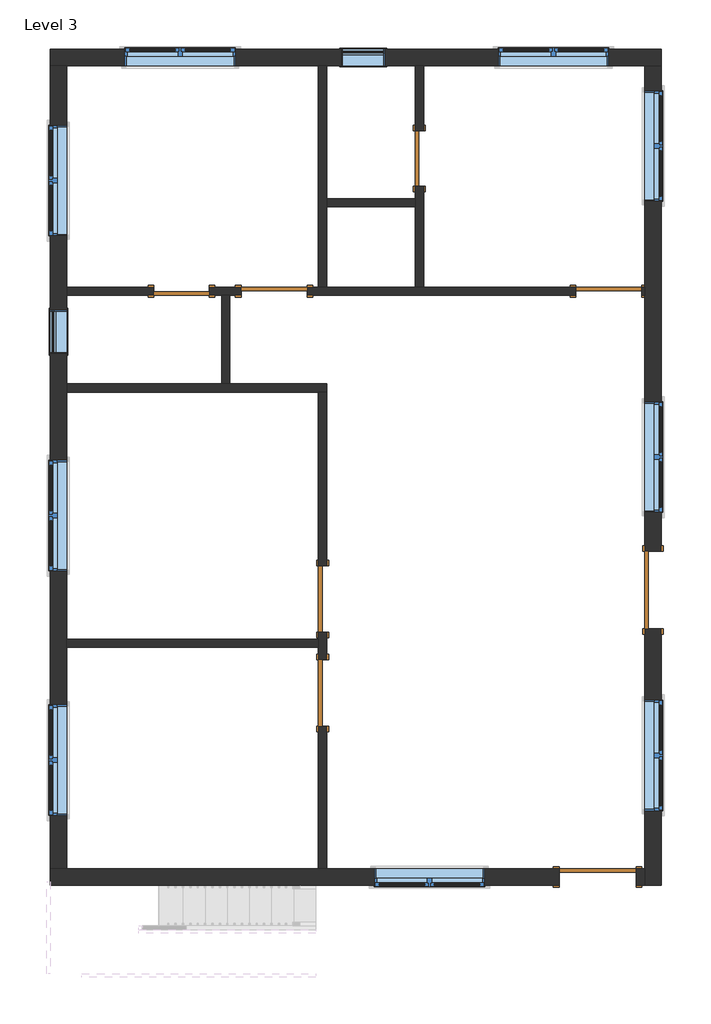
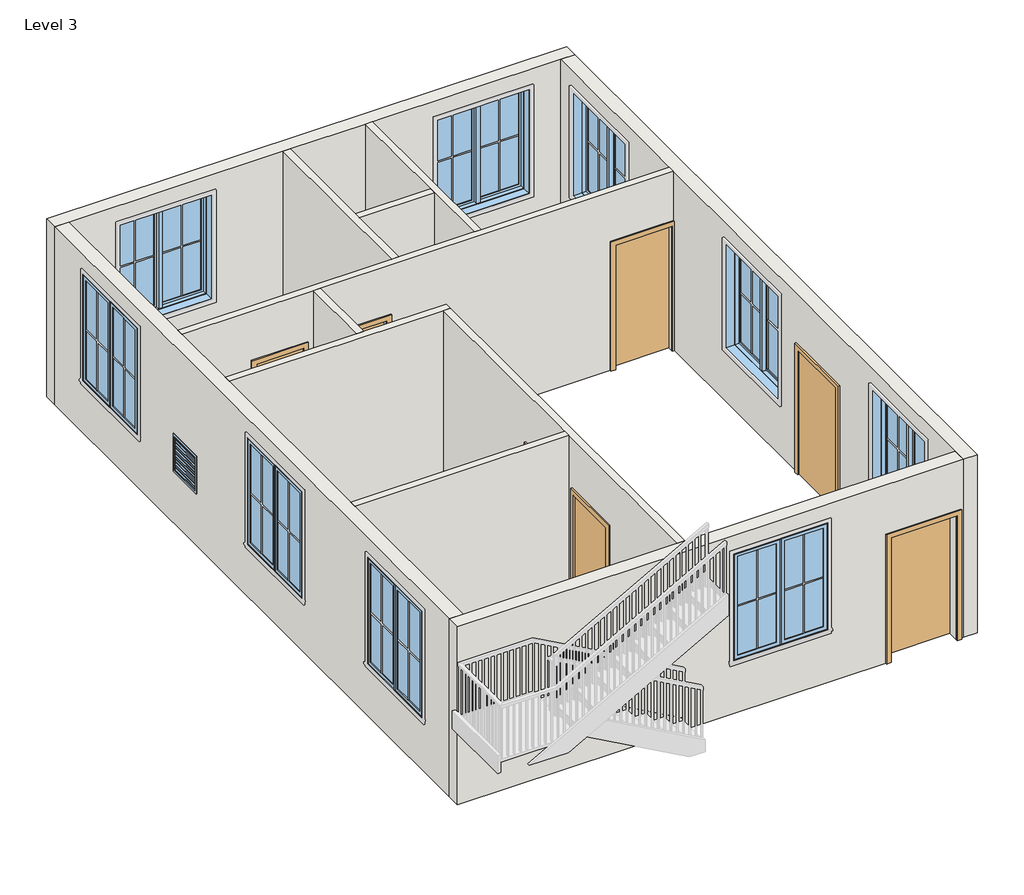
# One storey, part 1 of 3: 12 walls, 11 windows, 8 doors.
"""IFC4 building model written with IfcOpenShell, lengths in millimetres."""

from ifc_helpers import new_model, si_unit, frame, origin, place, context, project, spatial, polyline, outline, extrude, faceted_brep, transform, mapped, element, save
from components import door_78caadf7, single_flush_door_3_e5f9f3c4, single_flush_door_3_305aa2a5, door_9d399b00, door_0848dd25, window_casement_double_win_5_f93960c7, window_f2d8fef0

model = new_model("IFC4")

# Units and contexts
model_context = context("Model", 3, world=origin())
ifc_project = project(units=[si_unit("LENGTHUNIT", "METRE", prefix="MILLI")], contexts=[model_context])

# Site, building, storey
site = spatial("IfcSite", under=ifc_project)
building = spatial("IfcBuilding", under=site)
storey = spatial("IfcBuildingStorey", under=building, Name="Level 3", Elevation=3200.4)

# Doors
placement = place(None, origin())
door_shape = door_78caadf7(model_context)
element("IfcDoor", 1, ObjectType="Single-Flush : DOOR 2'6\"", at=placement, inside=storey, context=model_context, shape_type="MappedRepresentation", body=[
    mapped(door_shape, transform((-377.1698569, 4707.5566963, 3200.4), x_axis=(0.0, -1.0, 0.0), y_axis=(1.0, 0.0, 0.0), z_axis=(0.0, 0.0, 1.0))),
])
element("IfcDoor", 2, ObjectType="Single-Flush : DOOR 2'6\"", at=placement, inside=storey, context=model_context, shape_type="MappedRepresentation", body=[
    mapped(door_shape, transform((-3653.7698569, 2878.7566963, 3200.4), x_axis=(1.0, 0.0, 0.0), y_axis=(0.0, 1.0, 0.0), z_axis=(0.0, 0.0, 1.0))),
])
single_flush_door_3_shape = single_flush_door_3_e5f9f3c4(model_context)
element("IfcDoor", 3, ObjectType="Single-Flush : DOOR 3'", at=placement, inside=storey, context=model_context, shape_type="MappedRepresentation", body=[
    mapped(single_flush_door_3_shape, transform((-2377.4198569, 2878.7566963, 3200.4), x_axis=(1.0, 0.0, 0.0), y_axis=(0.0, 1.0, 0.0), z_axis=(0.0, 0.0, 1.0))),
])
element("IfcDoor", 4, ObjectType="Single-Flush : DOOR 3'", at=placement, inside=storey, context=model_context, shape_type="MappedRepresentation", body=[
    mapped(single_flush_door_3_shape, transform((2232.6801431, 2878.7566963, 3200.4), x_axis=(1.0, 0.0, 0.0), y_axis=(0.0, 1.0, 0.0), z_axis=(0.0, 0.0, 1.0))),
])
element("IfcDoor", 5, ObjectType="Single-Flush : DOOR 3'", at=placement, inside=storey, context=model_context, shape_type="MappedRepresentation", body=[
    mapped(single_flush_door_3_shape, transform((-1710.6698569, -2658.4433037, 3200.4), x_axis=(0.0, 1.0, 0.0), y_axis=(-1.0, 0.0, 0.0), z_axis=(0.0, 0.0, 1.0))),
])
single_flush_door_3_2_shape = single_flush_door_3_305aa2a5(model_context)
element("IfcDoor", 6, ObjectType="Single-Flush : DOOR 3'", at=placement, inside=storey, context=model_context, shape_type="MappedRepresentation", body=[
    mapped(single_flush_door_3_2_shape, transform((-1710.6698569, -1363.0433037, 3200.4), x_axis=(0.0, -1.0, 0.0), y_axis=(1.0, 0.0, 0.0), z_axis=(0.0, 0.0, 1.0))),
])
door_2_shape = door_9d399b00(model_context)
element("IfcDoor", 7, ObjectType="Single-Flush : DOOR 3'6\"", at=placement, inside=storey, context=model_context, shape_type="MappedRepresentation", body=[
    mapped(door_2_shape, transform((2080.2801431, -5192.0933037, 3200.4), x_axis=(1.0, 0.0, 0.0), y_axis=(0.0, 1.0, 0.0), z_axis=(0.0, 0.0, 1.0))),
])
door_3_shape = door_0848dd25(model_context)
element("IfcDoor", 8, ObjectType="Single-Flush : DOOR 3'6\"", at=placement, inside=storey, context=model_context, shape_type="MappedRepresentation", body=[
    mapped(door_3_shape, transform((2842.2801431, -1236.0433037, 3200.4), x_axis=(0.0, -1.0, 0.0), y_axis=(1.0, 0.0, 0.0), z_axis=(0.0, 0.0, 1.0))),
])

# Walls
element("IfcWall", 9, ObjectType="WALL 4.5\"", at=placement, inside=storey, context=model_context, shape_type="Brep", body=[
    faceted_brep([(2689.8801431, 2821.6066963, 5334.0), (2689.8801431, 2821.6066963, 3200.4), (2727.9801431, 2821.6066963, 3200.4), (2727.9801431, 2821.6066963, 6248.4), (-2987.0198569, 2821.6066963, 6248.4), (-3101.3198569, 2821.6066963, 6248.4), (-5234.9198569, 2821.6066963, 6248.4), (-5234.9198569, 2821.6066963, 3200.4), (-4034.7698569, 2821.6066963, 3200.4), (-4034.7698569, 2821.6066963, 5334.0), (-3272.7698569, 2821.6066963, 5334.0), (-3272.7698569, 2821.6066963, 3200.4), (-3101.3198569, 2821.6066963, 3200.4), (-2987.0198569, 2821.6066963, 3200.4), (-2834.6198569, 2821.6066963, 3200.4), (-2834.6198569, 2821.6066963, 5334.0), (-1920.2198569, 2821.6066963, 5334.0), (-1920.2198569, 2821.6066963, 3200.4), (1775.4801431, 2821.6066963, 3200.4), (1775.4801431, 2821.6066963, 5334.0), (2727.9801431, 2935.9066963, 3200.4), (2689.8801431, 2935.9066963, 3200.4), (2689.8801431, 2935.9066963, 5334.0), (1775.4801431, 2935.9066963, 5334.0), (1775.4801431, 2935.9066963, 3200.4), (-320.0198569, 2935.9066963, 3200.4), (-434.3198569, 2935.9066963, 3200.4), (-1653.5198569, 2935.9066963, 3200.4), (-1767.8198569, 2935.9066963, 3200.4), (-1920.2198569, 2935.9066963, 3200.4), (-1920.2198569, 2935.9066963, 5334.0), (-2834.6198569, 2935.9066963, 5334.0), (-2834.6198569, 2935.9066963, 3200.4), (-3272.7698569, 2935.9066963, 3200.4), (-3272.7698569, 2935.9066963, 5334.0), (-4034.7698569, 2935.9066963, 5334.0), (-4034.7698569, 2935.9066963, 3200.4), (-5234.9198569, 2935.9066963, 3200.4), (-5234.9198569, 2935.9066963, 6248.4), (-1767.8198569, 2935.9066963, 6248.4), (-1653.5198569, 2935.9066963, 6248.4), (-434.3198569, 2935.9066963, 6248.4), (-320.0198569, 2935.9066963, 6248.4), (2727.9801431, 2935.9066963, 6248.4)], [[[0, 1, 2, 3, 4, 5, 6, 7, 8, 9, 10, 11, 12, 13, 14, 15, 16, 17, 18, 19]], [[20, 21, 22, 23, 24, 25, 26, 27, 28, 29, 30, 31, 32, 33, 34, 35, 36, 37, 38, 39, 40, 41, 42, 43]], [[8, 7, 37, 36]], [[14, 13, 12, 11, 33, 32]], [[18, 17, 29, 28, 27, 26, 25, 24]], [[2, 1, 21, 20]], [[3, 2, 20, 43]], [[7, 6, 38, 37]], [[34, 33, 11, 10]], [[35, 34, 10, 9]], [[36, 35, 9, 8]], [[30, 29, 17, 16]], [[31, 30, 16, 15]], [[32, 31, 15, 14]], [[22, 21, 1, 0]], [[23, 22, 0, 19]], [[24, 23, 19, 18]], [[6, 5, 4, 3, 43, 42, 41, 40, 39, 38]]]),
])
element("IfcWall", 10, ObjectType="WALL 4.5\"", at=placement, inside=storey, context=model_context, shape_type="Brep", body=[
    faceted_brep([(-1767.8198569, 5983.9066963, 3200.4), (-1767.8198569, 2935.9066963, 3200.4), (-1767.8198569, 2935.9066963, 6248.4), (-1767.8198569, 5983.9066963, 6248.4), (-1653.5198569, 5983.9066963, 3200.4), (-1653.5198569, 5983.9066963, 6248.4), (-1653.5198569, 4155.1066963, 6248.4), (-1653.5198569, 4040.8066963, 6248.4), (-1653.5198569, 2935.9066963, 6248.4), (-1653.5198569, 2935.9066963, 3200.4), (-1653.5198569, 4040.8066963, 3200.4), (-1653.5198569, 4155.1066963, 3200.4)], [[[0, 1, 2, 3]], [[4, 5, 6, 7, 8, 9, 10, 11]], [[1, 0, 4, 11, 10, 9]], [[0, 3, 5, 4]], [[2, 1, 9, 8]], [[3, 2, 8, 7, 6, 5]]]),
])
element("IfcWall", 11, ObjectType="WALL 4.5\"", at=placement, inside=storey, context=model_context, shape_type="Brep", body=[
    faceted_brep([(-320.0198569, 2935.9066963, 3200.4), (-320.0198569, 4326.5566963, 3200.4), (-320.0198569, 4326.5566963, 5334.0), (-320.0198569, 5088.5566963, 5334.0), (-320.0198569, 5088.5566963, 3200.4), (-320.0198569, 5983.9066963, 3200.4), (-320.0198569, 5983.9066963, 6248.4), (-320.0198569, 2935.9066963, 6248.4), (-434.3198569, 4326.5566963, 5334.0), (-434.3198569, 4326.5566963, 3200.4), (-434.3198569, 4155.1066963, 3200.4), (-434.3198569, 4040.8066963, 3200.4), (-434.3198569, 2935.9066963, 3200.4), (-434.3198569, 2935.9066963, 6248.4), (-434.3198569, 4040.8066963, 6248.4), (-434.3198569, 4155.1066963, 6248.4), (-434.3198569, 5983.9066963, 6248.4), (-434.3198569, 5983.9066963, 3200.4), (-434.3198569, 5088.5566963, 3200.4), (-434.3198569, 5088.5566963, 5334.0)], [[[0, 1, 2, 3, 4, 5, 6, 7]], [[8, 9, 10, 11, 12, 13, 14, 15, 16, 17, 18, 19]], [[18, 17, 5, 4]], [[12, 11, 10, 9, 1, 0]], [[6, 5, 17, 16]], [[0, 7, 13, 12]], [[2, 1, 9, 8]], [[3, 2, 8, 19]], [[4, 3, 19, 18]], [[7, 6, 16, 15, 14, 13]]]),
])
element("IfcWall", 12, ObjectType="WALL 4.5\"", at=placement, inside=storey, context=model_context, shape_type="SweptSolid", body=[
    extrude(outline(polyline([(-434.3198569, 4040.8066963), (-1653.5198569, 4040.8066963), (-1653.5198569, 4155.1066963), (-434.3198569, 4155.1066963), (-434.3198569, 4040.8066963)])), frame((0.0, 0.0, 3200.4), z_axis=(0.0, 0.0, 1.0), x_axis=(1.0, 0.0, 0.0)), (0.0, 0.0, 1.0), 3048.0),
])
element("IfcWall", 13, ObjectType="WALL 4.5\"", at=placement, inside=storey, context=model_context, shape_type="Brep", body=[
    faceted_brep([(-5234.9198569, 1488.1066963, 3200.4), (-1767.8198569, 1488.1066963, 3200.4), (-1653.5198569, 1488.1066963, 3200.4), (-1653.5198569, 1488.1066963, 6248.4), (-1767.8198569, 1488.1066963, 6248.4), (-5234.9198569, 1488.1066963, 6248.4), (-5234.9198569, 1602.4066963, 3200.4), (-5234.9198569, 1602.4066963, 6248.4), (-3101.3198569, 1602.4066963, 6248.4), (-2987.0198569, 1602.4066963, 6248.4), (-1653.5198569, 1602.4066963, 6248.4), (-1653.5198569, 1602.4066963, 3200.4), (-2987.0198569, 1602.4066963, 3200.4), (-3101.3198569, 1602.4066963, 3200.4)], [[[0, 1, 2, 3, 4, 5]], [[6, 7, 8, 9, 10, 11, 12, 13]], [[2, 1, 0, 6, 13, 12, 11]], [[0, 5, 7, 6]], [[3, 2, 11, 10]], [[5, 4, 3, 10, 9, 8, 7]]]),
])
element("IfcWall", 14, ObjectType="WALL 4.5\"", at=placement, inside=storey, context=model_context, shape_type="Brep", body=[
    faceted_brep([(-1767.8198569, -1820.2433037, 3200.4), (-1767.8198569, -1915.4933037, 3200.4), (-1767.8198569, -2029.7933037, 3200.4), (-1767.8198569, -2201.2433037, 3200.4), (-1767.8198569, -2201.2433037, 5334.0), (-1767.8198569, -3115.6433037, 5334.0), (-1767.8198569, -3115.6433037, 3200.4), (-1767.8198569, -5077.7933037, 3200.4), (-1767.8198569, -5077.7933037, 6248.4), (-1767.8198569, -2029.7933037, 6248.4), (-1767.8198569, -1915.4933037, 6248.4), (-1767.8198569, 1488.1066963, 6248.4), (-1767.8198569, 1488.1066963, 3200.4), (-1767.8198569, -905.8433037, 3200.4), (-1767.8198569, -905.8433037, 5334.0), (-1767.8198569, -1820.2433037, 5334.0), (-1653.5198569, -2201.2433037, 5334.0), (-1653.5198569, -2201.2433037, 3200.4), (-1653.5198569, -1820.2433037, 3200.4), (-1653.5198569, -1820.2433037, 5334.0), (-1653.5198569, -905.8433037, 5334.0), (-1653.5198569, -905.8433037, 3200.4), (-1653.5198569, 1488.1066963, 3200.4), (-1653.5198569, 1488.1066963, 6248.4), (-1653.5198569, -5077.7933037, 6248.4), (-1653.5198569, -5077.7933037, 3200.4), (-1653.5198569, -3115.6433037, 3200.4), (-1653.5198569, -3115.6433037, 5334.0)], [[[0, 1, 2, 3, 4, 5, 6, 7, 8, 9, 10, 11, 12, 13, 14, 15]], [[16, 17, 18, 19, 20, 21, 22, 23, 24, 25, 26, 27]], [[13, 12, 22, 21]], [[26, 25, 7, 6]], [[18, 17, 3, 2, 1, 0]], [[12, 11, 23, 22]], [[8, 7, 25, 24]], [[19, 18, 0, 15]], [[20, 19, 15, 14]], [[21, 20, 14, 13]], [[4, 3, 17, 16]], [[5, 4, 16, 27]], [[6, 5, 27, 26]], [[11, 10, 9, 8, 24, 23]]]),
])
element("IfcWall", 15, ObjectType="WALL 4.5\"", at=placement, inside=storey, context=model_context, shape_type="SweptSolid", body=[
    extrude(outline(polyline([(-1767.8198569, -2029.7933037), (-5234.9198569, -2029.7933037), (-5234.9198569, -1915.4933037), (-1767.8198569, -1915.4933037), (-1767.8198569, -2029.7933037)])), frame((0.0, 0.0, 3200.4), z_axis=(0.0, 0.0, 1.0), x_axis=(1.0, 0.0, 0.0)), (0.0, 0.0, 1.0), 3048.0),
])
element("IfcWall", 16, ObjectType="WALL 4.5\"", at=placement, inside=storey, context=model_context, shape_type="SweptSolid", body=[
    extrude(outline(polyline([(-3101.3198569, 1602.4066963), (-3101.3198569, 2821.6066963), (-2987.0198569, 2821.6066963), (-2987.0198569, 1602.4066963), (-3101.3198569, 1602.4066963)])), frame((0.0, 0.0, 3200.4), z_axis=(0.0, 0.0, 1.0), x_axis=(1.0, 0.0, 0.0)), (0.0, 0.0, 1.0), 3048.0),
])
element("IfcWall", 17, ObjectType="WALL 9\"", at=placement, inside=storey, context=model_context, shape_type="Brep", body=[
    faceted_brep([(-5463.5198569, 5983.9066963, 3200.4), (-5234.9198569, 5983.9066963, 3200.4), (-1767.8198569, 5983.9066963, 3200.4), (-1653.5198569, 5983.9066963, 3200.4), (-434.3198569, 5983.9066963, 3200.4), (-320.0198569, 5983.9066963, 3200.4), (2727.9801431, 5983.9066963, 3200.4), (2956.5801431, 5983.9066963, 3200.4), (2956.5801431, 5983.9066963, 6248.4), (2727.9801431, 5983.9066963, 6248.4), (-320.0198569, 5983.9066963, 6248.4), (-434.3198569, 5983.9066963, 6248.4), (-1653.5198569, 5983.9066963, 6248.4), (-1767.8198569, 5983.9066963, 6248.4), (-5234.9198569, 5983.9066963, 6248.4), (-5463.5198569, 5983.9066963, 6248.4), (2232.6801431, 5983.9066963, 5943.6), (2232.6801431, 5983.9066963, 4114.8), (708.6801431, 5983.9066963, 4114.8), (708.6801431, 5983.9066963, 5943.6), (-2910.8198569, 5983.9066963, 5943.6), (-2910.8198569, 5983.9066963, 4114.8), (-4434.8198569, 5983.9066963, 4114.8), (-4434.8198569, 5983.9066963, 5943.6), (-1456.6698569, 5983.9066963, 4724.4), (-847.0698569, 5983.9066963, 4724.4), (-847.0698569, 5983.9066963, 4114.8), (-1456.6698569, 5983.9066963, 4114.8), (-5463.5198569, 6212.5066963, 3200.4), (-5463.5198569, 6212.5066963, 6248.4), (2956.5801431, 6212.5066963, 6248.4), (2956.5801431, 6212.5066963, 3200.4), (2232.6801431, 6212.5066963, 5943.6), (708.6801431, 6212.5066963, 5943.6), (708.6801431, 6212.5066963, 4114.8), (2232.6801431, 6212.5066963, 4114.8), (-2910.8198569, 6212.5066963, 5943.6), (-4434.8198569, 6212.5066963, 5943.6), (-4434.8198569, 6212.5066963, 4114.8), (-2910.8198569, 6212.5066963, 4114.8), (-1456.6698569, 6212.5066963, 4724.4), (-1456.6698569, 6212.5066963, 4114.8), (-847.0698569, 6212.5066963, 4114.8), (-847.0698569, 6212.5066963, 4724.4)], [[[0, 1, 2, 3, 4, 5, 6, 7, 8, 9, 10, 11, 12, 13, 14, 15], [16, 17, 18, 19], [20, 21, 22, 23], [24, 25, 26, 27]], [[28, 29, 30, 31], [32, 33, 34, 35], [36, 37, 38, 39], [40, 41, 42, 43]], [[7, 6, 5, 4, 3, 2, 1, 0, 28, 31]], [[8, 7, 31, 30]], [[0, 15, 29, 28]], [[17, 16, 32, 35]], [[18, 17, 35, 34]], [[19, 18, 34, 33]], [[16, 19, 33, 32]], [[21, 20, 36, 39]], [[22, 21, 39, 38]], [[23, 22, 38, 37]], [[20, 23, 37, 36]], [[41, 40, 24, 27]], [[42, 41, 27, 26]], [[43, 42, 26, 25]], [[40, 43, 25, 24]], [[15, 14, 13, 12, 11, 10, 9, 8, 30, 29]]]),
])
element("IfcWall", 18, ObjectType="WALL 9\"", at=placement, inside=storey, context=model_context, shape_type="Brep", body=[
    faceted_brep([(2727.9801431, -1769.4433037, 5334.0), (2727.9801431, -1769.4433037, 3200.4), (2727.9801431, -5077.7933037, 3200.4), (2727.9801431, -5306.3933037, 3200.4), (2727.9801431, -5306.3933037, 6248.4), (2727.9801431, -5077.7933037, 6248.4), (2727.9801431, 2821.6066963, 6248.4), (2727.9801431, 2935.9066963, 6248.4), (2727.9801431, 5983.9066963, 6248.4), (2727.9801431, 5983.9066963, 3200.4), (2727.9801431, 2935.9066963, 3200.4), (2727.9801431, 2821.6066963, 3200.4), (2727.9801431, -702.6433037, 3200.4), (2727.9801431, -702.6433037, 5334.0), (2727.9801431, 4117.0066963, 5943.6), (2727.9801431, 4117.0066963, 4114.8), (2727.9801431, 5641.0066963, 4114.8), (2727.9801431, 5641.0066963, 5943.6), (2727.9801431, -169.2433037, 5943.6), (2727.9801431, -169.2433037, 4114.8), (2727.9801431, 1354.7566963, 4114.8), (2727.9801431, 1354.7566963, 5943.6), (2727.9801431, -4277.6933037, 5943.6), (2727.9801431, -4277.6933037, 4114.8), (2727.9801431, -2753.6933037, 4114.8), (2727.9801431, -2753.6933037, 5943.6), (2956.5801431, -5306.3933037, 3200.4), (2956.5801431, -1769.4433037, 3200.4), (2956.5801431, -1769.4433037, 5334.0), (2956.5801431, -702.6433037, 5334.0), (2956.5801431, -702.6433037, 3200.4), (2956.5801431, 5983.9066963, 3200.4), (2956.5801431, 5983.9066963, 6248.4), (2956.5801431, -5306.3933037, 6248.4), (2956.5801431, 4117.0066963, 5943.6), (2956.5801431, 5641.0066963, 5943.6), (2956.5801431, 5641.0066963, 4114.8), (2956.5801431, 4117.0066963, 4114.8), (2956.5801431, -169.2433037, 5943.6), (2956.5801431, 1354.7566963, 5943.6), (2956.5801431, 1354.7566963, 4114.8), (2956.5801431, -169.2433037, 4114.8), (2956.5801431, -4277.6933037, 5943.6), (2956.5801431, -2753.6933037, 5943.6), (2956.5801431, -2753.6933037, 4114.8), (2956.5801431, -4277.6933037, 4114.8)], [[[0, 1, 2, 3, 4, 5, 6, 7, 8, 9, 10, 11, 12, 13], [14, 15, 16, 17], [18, 19, 20, 21], [22, 23, 24, 25]], [[26, 27, 28, 29, 30, 31, 32, 33], [34, 35, 36, 37], [38, 39, 40, 41], [42, 43, 44, 45]], [[3, 2, 1, 27, 26]], [[12, 11, 10, 9, 31, 30]], [[9, 8, 32, 31]], [[4, 3, 26, 33]], [[15, 14, 34, 37]], [[16, 15, 37, 36]], [[17, 16, 36, 35]], [[14, 17, 35, 34]], [[19, 18, 38, 41]], [[20, 19, 41, 40]], [[21, 20, 40, 39]], [[18, 21, 39, 38]], [[23, 22, 42, 45]], [[24, 23, 45, 44]], [[25, 24, 44, 43]], [[22, 25, 43, 42]], [[28, 27, 1, 0]], [[29, 28, 0, 13]], [[30, 29, 13, 12]], [[8, 7, 6, 5, 4, 33, 32]]]),
])
element("IfcWall", 19, ObjectType="WALL 9\"", at=placement, inside=storey, context=model_context, shape_type="Brep", body=[
    faceted_brep([(2727.9801431, -5077.7933037, 3200.4), (2613.6801431, -5077.7933037, 3200.4), (2613.6801431, -5077.7933037, 5334.0), (1546.8801431, -5077.7933037, 5334.0), (1546.8801431, -5077.7933037, 3200.4), (-1653.5198569, -5077.7933037, 3200.4), (-1767.8198569, -5077.7933037, 3200.4), (-5234.9198569, -5077.7933037, 3200.4), (-5463.5198569, -5077.7933037, 3200.4), (-5463.5198569, -5077.7933037, 6248.4), (-5234.9198569, -5077.7933037, 6248.4), (-1767.8198569, -5077.7933037, 6248.4), (-1653.5198569, -5077.7933037, 6248.4), (2727.9801431, -5077.7933037, 6248.4), (-999.4698569, -5077.7933037, 5943.6), (-999.4698569, -5077.7933037, 4114.8), (524.5301431, -5077.7933037, 4114.8), (524.5301431, -5077.7933037, 5943.6), (2613.6801431, -5306.3933037, 5334.0), (2613.6801431, -5306.3933037, 3200.4), (2727.9801431, -5306.3933037, 3200.4), (2727.9801431, -5306.3933037, 6248.4), (-1831.3198569, -5306.3933037, 6248.4), (-5463.5198569, -5306.3933037, 6248.4), (-5463.5198569, -5306.3933037, 3200.4), (1546.8801431, -5306.3933037, 3200.4), (1546.8801431, -5306.3933037, 5334.0), (-999.4698569, -5306.3933037, 5943.6), (524.5301431, -5306.3933037, 5943.6), (524.5301431, -5306.3933037, 4114.8), (-999.4698569, -5306.3933037, 4114.8)], [[[0, 1, 2, 3, 4, 5, 6, 7, 8, 9, 10, 11, 12, 13], [14, 15, 16, 17]], [[18, 19, 20, 21, 22, 23, 24, 25, 26], [27, 28, 29, 30]], [[25, 24, 8, 7, 6, 5, 4]], [[20, 19, 1, 0]], [[0, 13, 21, 20]], [[9, 8, 24, 23]], [[15, 14, 27, 30]], [[16, 15, 30, 29]], [[17, 16, 29, 28]], [[14, 17, 28, 27]], [[2, 1, 19, 18]], [[3, 2, 18, 26]], [[4, 3, 26, 25]], [[13, 12, 11, 10, 9, 23, 22, 21]]]),
])
element("IfcWall", 20, ObjectType="WALL 9\"", at=placement, inside=storey, context=model_context, shape_type="Brep", body=[
    faceted_brep([(-5234.9198569, -5077.7933037, 3200.4), (-5234.9198569, -2029.7933037, 3200.4), (-5234.9198569, -1915.4933037, 3200.4), (-5234.9198569, 1488.1066963, 3200.4), (-5234.9198569, 1602.4066963, 3200.4), (-5234.9198569, 2821.6066963, 3200.4), (-5234.9198569, 2935.9066963, 3200.4), (-5234.9198569, 5983.9066963, 3200.4), (-5234.9198569, 5983.9066963, 6248.4), (-5234.9198569, 2935.9066963, 6248.4), (-5234.9198569, 2821.6066963, 6248.4), (-5234.9198569, 1602.4066963, 6248.4), (-5234.9198569, 1488.1066963, 6248.4), (-5234.9198569, -1915.4933037, 6248.4), (-5234.9198569, -2029.7933037, 6248.4), (-5234.9198569, -5077.7933037, 6248.4), (-5234.9198569, -2820.3683037, 5943.6), (-5234.9198569, -2820.3683037, 4114.8), (-5234.9198569, -4344.3683037, 4114.8), (-5234.9198569, -4344.3683037, 5943.6), (-5234.9198569, 548.3066963, 5943.6), (-5234.9198569, 548.3066963, 4114.8), (-5234.9198569, -975.6933037, 4114.8), (-5234.9198569, -975.6933037, 5943.6), (-5234.9198569, 5164.7566963, 5943.6), (-5234.9198569, 5164.7566963, 4114.8), (-5234.9198569, 3640.7566963, 4114.8), (-5234.9198569, 3640.7566963, 5943.6), (-5234.9198569, 2015.1566963, 4724.4), (-5234.9198569, 2624.7566963, 4724.4), (-5234.9198569, 2624.7566963, 4114.8), (-5234.9198569, 2015.1566963, 4114.8), (-5463.5198569, -5077.7933037, 3200.4), (-5463.5198569, -5077.7933037, 6248.4), (-5463.5198569, 5983.9066963, 6248.4), (-5463.5198569, 5983.9066963, 3200.4), (-5463.5198569, -2820.3683037, 5943.6), (-5463.5198569, -4344.3683037, 5943.6), (-5463.5198569, -4344.3683037, 4114.8), (-5463.5198569, -2820.3683037, 4114.8), (-5463.5198569, 548.3066963, 5943.6), (-5463.5198569, -975.6933037, 5943.6), (-5463.5198569, -975.6933037, 4114.8), (-5463.5198569, 548.3066963, 4114.8), (-5463.5198569, 5164.7566963, 5943.6), (-5463.5198569, 3640.7566963, 5943.6), (-5463.5198569, 3640.7566963, 4114.8), (-5463.5198569, 5164.7566963, 4114.8), (-5463.5198569, 2015.1566963, 4724.4), (-5463.5198569, 2015.1566963, 4114.8), (-5463.5198569, 2624.7566963, 4114.8), (-5463.5198569, 2624.7566963, 4724.4)], [[[0, 1, 2, 3, 4, 5, 6, 7, 8, 9, 10, 11, 12, 13, 14, 15], [16, 17, 18, 19], [20, 21, 22, 23], [24, 25, 26, 27], [28, 29, 30, 31]], [[32, 33, 34, 35], [36, 37, 38, 39], [40, 41, 42, 43], [44, 45, 46, 47], [48, 49, 50, 51]], [[7, 6, 5, 4, 3, 2, 1, 0, 32, 35]], [[8, 7, 35, 34]], [[0, 15, 33, 32]], [[17, 16, 36, 39]], [[18, 17, 39, 38]], [[19, 18, 38, 37]], [[16, 19, 37, 36]], [[21, 20, 40, 43]], [[22, 21, 43, 42]], [[23, 22, 42, 41]], [[20, 23, 41, 40]], [[25, 24, 44, 47]], [[26, 25, 47, 46]], [[27, 26, 46, 45]], [[24, 27, 45, 44]], [[49, 48, 28, 31]], [[50, 49, 31, 30]], [[51, 50, 30, 29]], [[48, 51, 29, 28]], [[15, 14, 13, 12, 11, 10, 9, 8, 34, 33]]]),
])

# Windows
window_casement_double_win_5_shape = window_casement_double_win_5_f93960c7(model_context)
element("IfcWindow", 21, ObjectType="Window-Casement-Double : WIN 5'", at=placement, inside=storey, context=model_context, shape_type="MappedRepresentation", body=[
    mapped(window_casement_double_win_5_shape, transform((-5349.2198569, -3582.3683037, 3200.4), x_axis=(0.0, 1.0, 0.0), y_axis=(-1.0, 0.0, 0.0), z_axis=(0.0, 0.0, 1.0))),
])
element("IfcWindow", 22, ObjectType="Window-Casement-Double : WIN 5'", at=placement, inside=storey, context=model_context, shape_type="MappedRepresentation", body=[
    mapped(window_casement_double_win_5_shape, transform((-5349.2198569, -213.6933037, 3200.4), x_axis=(0.0, 1.0, 0.0), y_axis=(-1.0, 0.0, 0.0), z_axis=(0.0, 0.0, 1.0))),
])
element("IfcWindow", 23, ObjectType="Window-Casement-Double : WIN 5'", at=placement, inside=storey, context=model_context, shape_type="MappedRepresentation", body=[
    mapped(window_casement_double_win_5_shape, transform((-5349.2198569, 4402.7566963, 3200.4), x_axis=(0.0, 1.0, 0.0), y_axis=(-1.0, 0.0, 0.0), z_axis=(0.0, 0.0, 1.0))),
])
element("IfcWindow", 24, ObjectType="Window-Casement-Double : WIN 5'", at=placement, inside=storey, context=model_context, shape_type="MappedRepresentation", body=[
    mapped(window_casement_double_win_5_shape, transform((2842.2801431, 4879.0066963, 3200.4), x_axis=(0.0, -1.0, 0.0), y_axis=(1.0, 0.0, 0.0), z_axis=(0.0, 0.0, 1.0))),
])
element("IfcWindow", 25, ObjectType="Window-Casement-Double : WIN 5'", at=placement, inside=storey, context=model_context, shape_type="MappedRepresentation", body=[
    mapped(window_casement_double_win_5_shape, transform((2842.2801431, 592.7566963, 3200.4), x_axis=(0.0, -1.0, 0.0), y_axis=(1.0, 0.0, 0.0), z_axis=(0.0, 0.0, 1.0))),
])
element("IfcWindow", 26, ObjectType="Window-Casement-Double : WIN 5'", at=placement, inside=storey, context=model_context, shape_type="MappedRepresentation", body=[
    mapped(window_casement_double_win_5_shape, transform((2842.2801431, -3515.6933037, 3200.4), x_axis=(0.0, -1.0, 0.0), y_axis=(1.0, 0.0, 0.0), z_axis=(0.0, 0.0, 1.0))),
])
element("IfcWindow", 27, ObjectType="Window-Casement-Double : WIN 5'", at=placement, inside=storey, context=model_context, shape_type="MappedRepresentation", body=[
    mapped(window_casement_double_win_5_shape, transform((-237.4698569, -5192.0933037, 3200.4), x_axis=(-1.0, 0.0, 0.0), y_axis=(0.0, -1.0, 0.0), z_axis=(0.0, 0.0, 1.0))),
])
element("IfcWindow", 28, ObjectType="Window-Casement-Double : WIN 5'", at=placement, inside=storey, context=model_context, shape_type="MappedRepresentation", body=[
    mapped(window_casement_double_win_5_shape, transform((1470.6801431, 6098.2066963, 3200.4), x_axis=(1.0, 0.0, 0.0), y_axis=(0.0, 1.0, 0.0), z_axis=(0.0, 0.0, 1.0))),
])
element("IfcWindow", 29, ObjectType="Window-Casement-Double : WIN 5'", at=placement, inside=storey, context=model_context, shape_type="MappedRepresentation", body=[
    mapped(window_casement_double_win_5_shape, transform((-3672.8198569, 6098.2066963, 3200.4), x_axis=(1.0, 0.0, 0.0), y_axis=(0.0, 1.0, 0.0), z_axis=(0.0, 0.0, 1.0))),
])
window_shape = window_f2d8fef0(model_context)
element("IfcWindow", 30, ObjectType="Window-Louvers : 24\" x 24\"", at=placement, inside=storey, context=model_context, shape_type="MappedRepresentation", body=[
    mapped(window_shape, transform((-1151.8698569, 6104.5566963, 3200.4), x_axis=(1.0, 0.0, 0.0), y_axis=(0.0, 1.0, 0.0), z_axis=(0.0, 0.0, 1.0))),
])
element("IfcWindow", 31, ObjectType="Window-Louvers : 24\" x 24\"", at=placement, inside=storey, context=model_context, shape_type="MappedRepresentation", body=[
    mapped(window_shape, transform((-5355.5698569, 2319.9566963, 3200.4), x_axis=(0.0, 1.0, 0.0), y_axis=(-1.0, 0.0, 0.0), z_axis=(0.0, 0.0, 1.0))),
])

save(model, "model.ifc")

# Revit data of these elements
# Type "Single-Flush : DOOR 2'6\""
#   Type Mark = "10"
#   Construction Type Id = "MDOOR"
#   Assembly Code = "C1020"
#   Analytic Construction = "Metal"
#   Thickness = 0' - 2"
#   Heat Transfer Coefficient (U) = 0.651978 BTU/(h·ft²·°F)
#   Height = 7' - 0"
#   Trim Projection Ext = 0' - 1"
#   Trim Projection Int = 0' - 1"
#   Trim Width = 0' - 3"
#   Width = 2' - 6"
#   Define Thermal Properties by = 1
#   Door Material = Door - Panel
#   Frame Material = Door - Frame
#   Visual Light Transmittance = 0
#   Solar Heat Gain Coefficient = 0
#   Function = (empty or 0)
#   Wall Closure = (empty or 0)
# Type "Single-Flush : DOOR 3'"
#   Type Mark = "8"
#   Construction Type Id = "MDOOR"
#   Assembly Code = "C1020"
#   Analytic Construction = "Metal"
#   Thickness = 0' - 2"
#   Heat Transfer Coefficient (U) = 0.651978 BTU/(h·ft²·°F)
#   Height = 7' - 0"
#   Trim Projection Ext = 0' - 1"
#   Trim Projection Int = 0' - 1"
#   Trim Width = 0' - 3"
#   Width = 3' - 0"
#   Define Thermal Properties by = 1
#   Door Material = Door - Panel
#   Frame Material = Door - Frame
#   Visual Light Transmittance = 0
#   Solar Heat Gain Coefficient = 0
#   Function = (empty or 0)
#   Wall Closure = (empty or 0)
# Type "Single-Flush : DOOR 3'6\""
#   Type Mark = "9"
#   Construction Type Id = "MDOOR"
#   Assembly Code = "C1020"
#   Analytic Construction = "Metal"
#   Thickness = 0' - 2"
#   Heat Transfer Coefficient (U) = 0.651978 BTU/(h·ft²·°F)
#   Height = 7' - 0"
#   Trim Projection Ext = 0' - 1"
#   Trim Projection Int = 0' - 1"
#   Trim Width = 0' - 3"
#   Width = 3' - 6"
#   Define Thermal Properties by = 1
#   Door Material = Door - Panel
#   Frame Material = Door - Frame
#   Visual Light Transmittance = 0
#   Solar Heat Gain Coefficient = 0
#   Function = (empty or 0)
#   Wall Closure = (empty or 0)
# Type "WALL 4.5\""
#   Assembly Code = "B2010"
#   Layers, outside or top first: 0' - 4 1/2" no material (function 1)
# Type "WALL 9\""
#   Assembly Code = "B2010"
#   Layers, outside or top first: 0' - 9" no material (function 1)
# Type "Window-Casement-Double : WIN 5'"
#   Type Mark = "20"
#   Fire Rating = "0.5h"
#   Assembly Code = "B2020100"
#   Analytic Construction = "Double glazing - domestic"
#   Frame Extension [instance default] = 0' - 0 1/4"
#   Window Inset [instance default] = 0' - 0"
#   Wall Thickness [instance default] = 0' - 6"
#   Interior Wall Closure [instance default] = 0' - 2 1/4"
#   Half Width = 2' - 6"
#   Visual Light Transmittance = 0.81
#   Thermal Resistance (R) = 1.8146 (h·ft²·°F)/BTU
#   Solar Heat Gain Coefficient = 0.76
#   Rough Width = 5' - 0 1/2"
#   Rough Height = 6' - 0 1/2"
#   Height = 6' - 0"
#   Heat Transfer Coefficient (U) = 0.5511 BTU/(h·ft²·°F)
#   Exterior Wall Closure [instance default] = 0' - 1 1/4"
#   Extension Jamb [instance default] = 0' - 2 1/4"
#   Default Sill Height = 3' - 0"
#   Width = 5' - 0"
#   Muntin Visibility = yes
#   Interior Trim Visibility [instance default] = yes
#   Exterior Trim Visibility [instance default] = yes
#   Extension Jamb Visibility [instance default] = yes
#   Interior Trim Material = Wood - Stained
#   Muntin Pattern = Muntin Pattern_2x2 : Muntin Pattern_2x2
#   Interior Trim = Trim-Window-Interior-Flat : Picture Frame
#   Interior Frame Material = Wood - Stained
#   Glass Panel Material = Glass
#   Exterior Trim Material = Clad - White
#   Exterior Trim = Trim-Window-Exterior-Flat : with Sill
#   Exterior Frame Material = Clad - White
#   Wall Closure = (empty or 0)
# Type "Window-Louvers : 24\" x 24\""
#   Type Mark = "21"
#   Construction Type Id = "GSP4R"
#   Assembly Code = "B20"
#   Analytic Construction = "1/8 in Pilkington single glazing"
#   Visual Light Transmittance = 0.9
#   Thermal Resistance (R) = 1.53941 (h·ft²·°F)/BTU
#   Solar Heat Gain Coefficient = 0.78
#   Max Height = 1' - 11.74264"
#   Height = 2' - 0"
#   Heat Transfer Coefficient (U) = 0.6496 BTU/(h·ft²·°F)
#   Blade Width [instance default] = 1' - 10 1/2"
#   Blade Vertical Thickness = 0' - 0.35355"
#   Blade Thickness = 0' - 0 1/4"
#   Blade Spacing = 0' - 1 1/2"
#   Blade Height = 0' - 1.85355"
#   Blade Depth = 0' - 3"
#   Blade Angle = 45.00°
#   Default Sill Height = 3' - 0"
#   Trim Projection_Exterior = 0' - 0 1/2"
#   Trim Projection_Interior = 0' - 0 1/2"
#   Trim Width_Exterior = 0' - 1 1/2"
#   Trim Width_Interior = 0' - 1 1/2"
#   Width = 2' - 0"
#   Max Blade Count = 12
#   Define Thermal Properties by = 1
#   Blade Count = 12
#   Frame Material = Birch
#   Louver Material = Birch
#   Trim Exterior Material = Birch
#   Trim Interior Material = Birch
#   Wall Closure = (empty or 0)
# Elements 1, 2 (IfcDoor, "Single-Flush : DOOR 2'6\"")
#   Phase Created = New Construction
#   Materials on its faces: "Door - Frame", "Door - Panel"
# Elements 3, 4, 5, 6 (IfcDoor, "Single-Flush : DOOR 3'")
#   Phase Created = New Construction
#   Materials on its faces: "Door - Frame", "Door - Panel"
# Elements 7, 8 (IfcDoor, "Single-Flush : DOOR 3'6\"")
#   Phase Created = New Construction
#   Materials on its faces: "Door - Frame", "Door - Panel"
# Elements 9, 10, 11, 12, 13, 14, 15, 16 (IfcWall, "WALL 4.5\"")
#   Top Offset = 0' - 0"
#   Base Offset = 0' - 0"
#   Unconnected Height = 10' - 0"
#   wall height = 10' - 0"
#   Phase Created = New Construction
#   Base Constraint = Level 3
#   Materials on its faces: "Default Wall"
# Elements 17, 18, 19, 20 (IfcWall, "WALL 9\"")
#   Top Offset = 0' - 0"
#   Base Offset = 0' - 0"
#   Unconnected Height = 10' - 0"
#   wall height = 10' - 0"
#   Phase Created = New Construction
#   Base Constraint = Level 3
#   Materials on its faces: "Default Wall", "Cherry"
# Element 21 (IfcWindow, "Window-Casement-Double : WIN 5'")
#   Mark = "12"
#   Window Inset = 0' - 0"
#   Interior Wall Closure = 0' - 2 1/4"
#   Frame Extension = 0' - 0 1/4"
#   Exterior Wall Closure = 0' - 1 1/4"
#   Interior Trim Visibility = yes
#   Exterior Trim Visibility = yes
#   Phase Created = New Construction
#   Materials on its faces: "Wood - Stained", "Glass", "Clad - White"
# Element 22 (IfcWindow, "Window-Casement-Double : WIN 5'")
#   Mark = "13"
#   Window Inset = 0' - 0"
#   Interior Wall Closure = 0' - 2 1/4"
#   Frame Extension = 0' - 0 1/4"
#   Exterior Wall Closure = 0' - 1 1/4"
#   Interior Trim Visibility = yes
#   Exterior Trim Visibility = yes
#   Phase Created = New Construction
#   Materials on its faces: "Wood - Stained", "Glass", "Clad - White"
# Element 23 (IfcWindow, "Window-Casement-Double : WIN 5'")
#   Mark = "14"
#   Window Inset = 0' - 0"
#   Interior Wall Closure = 0' - 2 1/4"
#   Frame Extension = 0' - 0 1/4"
#   Exterior Wall Closure = 0' - 1 1/4"
#   Interior Trim Visibility = yes
#   Exterior Trim Visibility = yes
#   Phase Created = New Construction
#   Materials on its faces: "Wood - Stained", "Glass", "Clad - White"
# Element 24 (IfcWindow, "Window-Casement-Double : WIN 5'")
#   Mark = "15"
#   Window Inset = 0' - 0"
#   Interior Wall Closure = 0' - 2 1/4"
#   Frame Extension = 0' - 0 1/4"
#   Exterior Wall Closure = 0' - 1 1/4"
#   Interior Trim Visibility = yes
#   Exterior Trim Visibility = yes
#   Phase Created = New Construction
#   Materials on its faces: "Wood - Stained", "Glass", "Clad - White"
# Element 25 (IfcWindow, "Window-Casement-Double : WIN 5'")
#   Mark = "16"
#   Window Inset = 0' - 0"
#   Interior Wall Closure = 0' - 2 1/4"
#   Frame Extension = 0' - 0 1/4"
#   Exterior Wall Closure = 0' - 1 1/4"
#   Interior Trim Visibility = yes
#   Exterior Trim Visibility = yes
#   Phase Created = New Construction
#   Materials on its faces: "Wood - Stained", "Glass", "Clad - White"
# Element 26 (IfcWindow, "Window-Casement-Double : WIN 5'")
#   Mark = "17"
#   Window Inset = 0' - 0"
#   Interior Wall Closure = 0' - 2 1/4"
#   Frame Extension = 0' - 0 1/4"
#   Exterior Wall Closure = 0' - 1 1/4"
#   Interior Trim Visibility = yes
#   Exterior Trim Visibility = yes
#   Phase Created = New Construction
#   Materials on its faces: "Wood - Stained", "Glass", "Clad - White"
# Element 27 (IfcWindow, "Window-Casement-Double : WIN 5'")
#   Mark = "18"
#   Window Inset = 0' - 0"
#   Interior Wall Closure = 0' - 2 1/4"
#   Frame Extension = 0' - 0 1/4"
#   Exterior Wall Closure = 0' - 1 1/4"
#   Interior Trim Visibility = yes
#   Exterior Trim Visibility = yes
#   Phase Created = New Construction
#   Materials on its faces: "Wood - Stained", "Glass", "Clad - White"
# Element 28 (IfcWindow, "Window-Casement-Double : WIN 5'")
#   Mark = "19"
#   Window Inset = 0' - 0"
#   Interior Wall Closure = 0' - 2 1/4"
#   Frame Extension = 0' - 0 1/4"
#   Exterior Wall Closure = 0' - 1 1/4"
#   Interior Trim Visibility = yes
#   Exterior Trim Visibility = yes
#   Phase Created = New Construction
#   Materials on its faces: "Wood - Stained", "Glass", "Clad - White"
# Element 29 (IfcWindow, "Window-Casement-Double : WIN 5'")
#   Mark = "20"
#   Window Inset = 0' - 0"
#   Interior Wall Closure = 0' - 2 1/4"
#   Frame Extension = 0' - 0 1/4"
#   Exterior Wall Closure = 0' - 1 1/4"
#   Interior Trim Visibility = yes
#   Exterior Trim Visibility = yes
#   Phase Created = New Construction
#   Materials on its faces: "Wood - Stained", "Glass", "Clad - White"
# Element 30 (IfcWindow, "Window-Louvers : 24\" x 24\"")
#   Mark = "21"
#   Blade Width = 1' - 10 1/2"
#   Phase Created = New Construction
#   Materials on its faces: "Birch"
# Element 31 (IfcWindow, "Window-Louvers : 24\" x 24\"")
#   Mark = "22"
#   Blade Width = 1' - 10 1/2"
#   Phase Created = New Construction
#   Materials on its faces: "Birch"
# Materials
#   "Door - Panel": class "Wood", colour RGB 210 159 95, transparency 0, Cost = 0
#   "Door - Frame": colour RGB 118 70 51, transparency 0, Cost = 0
#   "Wood - Stained": class "Wood", colour RGB 224 178 126, transparency 0, Cost = 0
#   "Glass": class "Glass", colour RGB 0 128 192, transparency 0.75, Description = "Soda Lime Glass", Cost = 0
#   "Clad - White": class "Wood", colour RGB 242 242 238, transparency 0, Cost = 0
#   "Birch": class "Wood", colour RGB 224 178 126, transparency 0, Description = "Betula Alleghaniensis", Cost = 0
#   "Default Wall": colour RGB 128 128 128, transparency 0, Cost = 0
#   "Cherry": class "Wood", colour RGB 226 177 128, transparency 0, Description = "Prunus Serotina", Cost = 0
